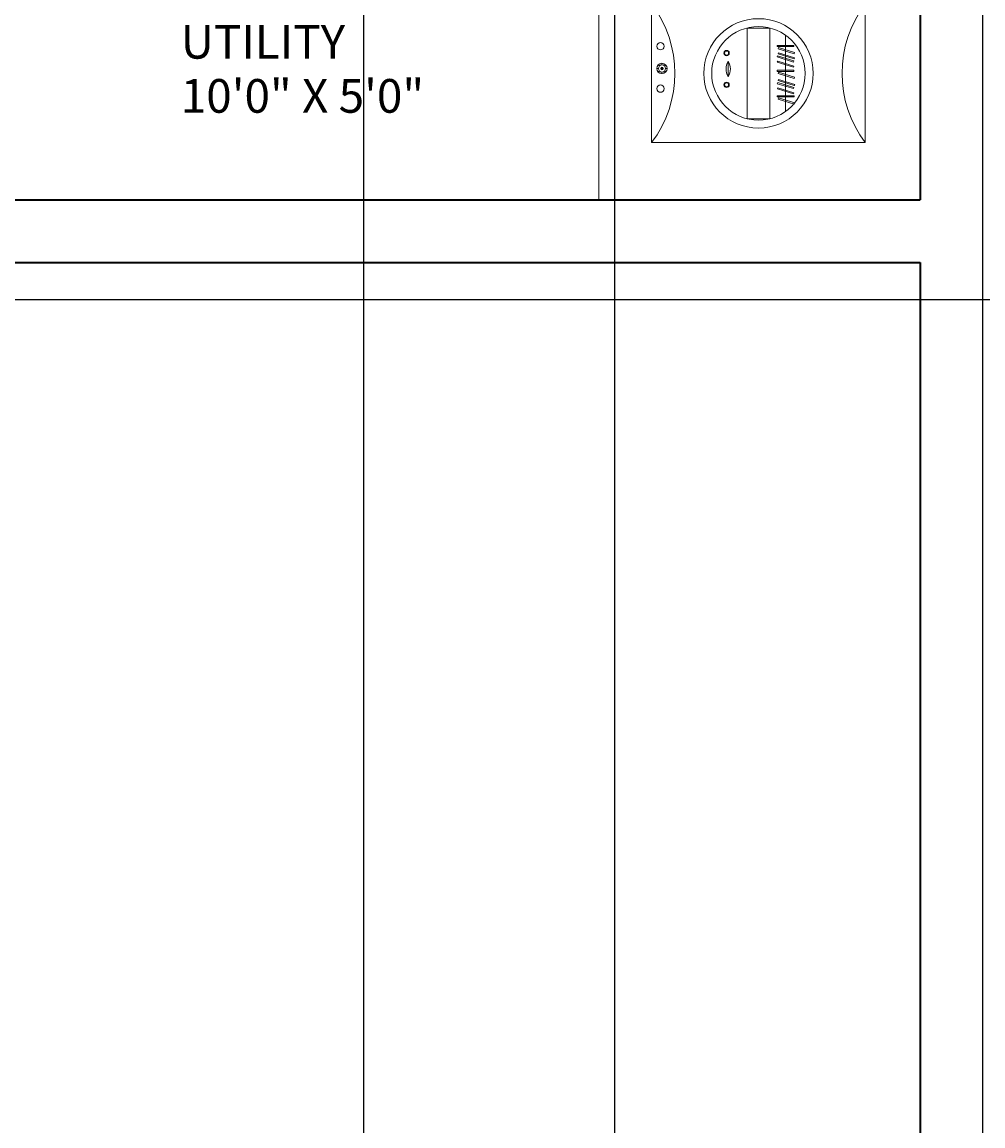
# Model space of a CAD drawing. Units: inches. Extents: x -61 to 1599, y -1316 to 257.
# Tile 81 of 204: x 407 to 545, y -565 to -407. Entities that reach past the tile are written whole.
import ezdxf

# ---------------------------------------------------------------- set-up
doc = ezdxf.new("R2010")
doc.units = ezdxf.units.IN
doc.header["$MEASUREMENT"] = 0
for name, color, linetype, lineweight in [('A-ANNO-DIMS', 2, 'Continuous', 18), ('A-AREA-IDEN', 1, 'Continuous', 18), ('A-EQPM', 9, 'Continuous', 18), ('A-FLOR-CASE', 8, 'Continuous', 18), ('WALLS', 4, 'Continuous', 35)]:
    doc.layers.add(name, color=color, linetype=linetype, lineweight=lineweight)
doc.styles.get("Standard").update_dxf_attribs({"font": 'arial.ttf'})
doc.dimstyles.get("Standard").update_dxf_attribs({"dimtxt": 0.18, "dimasz": 0.18, "dimexe": 0.18, "dimexo": 0.0625, "dimgap": 0.09, "dimtad": 0, "dimtih": 1, "dimtoh": 1, "dimdec": 0, "dimzin": 0, "dimdsep": 46, "dimlunit": 3, "dimtxsty": 'Standard', "dimcen": 0.09, "dimadec": 0, "dimazin": 0, "dimtfac": 1, "dimtdec": 0, "dimtofl": 0, "dimtmove": 0, "dimatfit": 3, "dimfxl": 1, "dimtolj": 1, "dimtzin": 0, "dimarcsym": 0})

# ---------------------------------------------------------------- blocks, each defined once
blk = doc.blocks.new('WASHING-MACHINE')
for p, q in [((19.24, 4.47), (19.22, 15.41)), ((0.96, 11.16), (1.13, 11)), ((1.49, 11.38), (1.49, 11.15)), ((2.02, 11.15), (1.86, 10.99)), ((11, 9.47), (11, 11.68)), ((0.98, 10.64), (0.75, 10.64)), ((1.12, 10.28), (0.96, 10.12)), ((1.49, 10.12), (1.49, 9.89)), ((1.86, 10.28), (2.02, 10.12)), ((2.23, 10.64), (2, 10.64))]:
    blk.add_line(p, q)
for points in [[(30.68, 0), (0, 0), (0, 19.87), (30.68, 19.87)], [(16.98, 3.42), (13.7, 3.42), (13.7, 16.45), (16.98, 16.45)], [(20.43, 13.78), (18.01, 13.78), (18.01, 13.95), (20.43, 13.95)], [(18.21, 13.64), (20.52, 12.92), (20.47, 12.76), (18.16, 13.47)], [(18.22, 12.89), (20.53, 12.18), (20.48, 12.01), (18.17, 12.73)], [(18.09, 12.45), (20.41, 11.74), (20.35, 11.57), (18.04, 12.29)], [(18.1, 11.71), (20.41, 10.99), (20.36, 10.83), (18.05, 11.54)], [(20.44, 10.23), (18.02, 10.23), (18.02, 10.4), (20.44, 10.4)], [(18.22, 10.09), (20.53, 9.38), (20.48, 9.21), (18.17, 9.92)], [(18.1, 8.63), (20.42, 7.91), (20.37, 7.75), (18.05, 8.46)], [(18.23, 9.07), (20.54, 8.36), (20.49, 8.19), (18.18, 8.91)], [(20.45, 6.56), (18.03, 6.56), (18.03, 6.73), (20.45, 6.73)], [(18.11, 7.88), (20.42, 7.17), (20.37, 7), (18.06, 7.72)], [(18.23, 6.42), (20.54, 5.7), (20.49, 5.54), (18.18, 6.25)]]:
    blk.add_lwpolyline(points, close=True)
for centre, radius in [((15.34, 9.94), 7.85), ((15.34, 9.94), 7.85), ((15.34, 9.94), 6.71), ((1.28, 13.83), 0.526), ((10.77, 12.86), 0.381), ((10.77, 12.86), 0.289), ((1.49, 10.64), 0.742), ((1.49, 10.64), 0.513), ((1.49, 10.64), 0.178), ((1.49, 10.64), 0.07), ((1.28, 7.75), 0.526), ((10.77, 8.29), 0.381), ((10.77, 8.29), 0.289)]:
    blk.add_circle(centre, radius)
for centre, radius, start, end in [((-13.12, 9.94), 16.46, 322.8671, 37.1329), ((43.8, 9.94), 16.46, 142.8671, 217.1329), ((12.8, 10.57), 2.11, 148.4251, 211.5749), ((9.2, 10.57), 2.11, 328.4251, 31.5749)]:
    blk.add_arc(centre, radius, start, end)
blk = doc.blocks.new('*D699')
at = {"layer": 'A-ANNO-DIMS', "color": 0, "lineweight": -2, "transparency": 16777216}
for p, q in [((835.64, -167.17), (-61.08, -167.17)), ((-60.9, -167.35), (-60.9, -306.73)), ((-60.9, -446.47), (-60.9, -307.09)), ((841.64, -446.65), (-61.08, -446.65))]:
    blk.add_line(p, q, dxfattribs=at)
at = {"layer": 'A-ANNO-DIMS', "color": 0, "transparency": 16777216}
for points in [[(-60.93, -167.35), (-60.87, -167.35), (-60.9, -167.17)], [(-60.93, -446.47), (-60.87, -446.47), (-60.9, -446.65)]]:
    blk.add_solid(points, dxfattribs=at)
at = {"layer": 'DEFPOINTS', "color": 0, "transparency": 16777216}
for p in [(835.7, -167.17), (-60.9, -446.65), (841.7, -446.65)]:
    blk.add_point(p, dxfattribs=at)
at = {"layer": 'A-ANNO-DIMS', "color": 0, "transparency": 16777216, "insert": (-60.9, -306.91), "char_height": 0.18, "attachment_point": 5}
blk.add_mtext('\\A1;279.5', dxfattribs=at)
blk = doc.blocks.new('*D703')
at = {"layer": 'A-ANNO-DIMS', "color": 0, "lineweight": -2, "transparency": 16777216}
for p, q in [((372.32, -616.88), (372.32, 257.46)), ((372.5, 257.28), (413.7, 257.28)), ((455.65, 257.28), (414.45, 257.28)), ((455.83, -616.88), (455.83, 257.46))]:
    blk.add_line(p, q, dxfattribs=at)
at = {"layer": 'A-ANNO-DIMS', "color": 0, "transparency": 16777216}
for points in [[(372.5, 257.31), (372.5, 257.25), (372.32, 257.28)], [(455.65, 257.31), (455.65, 257.25), (455.83, 257.28)]]:
    blk.add_solid(points, dxfattribs=at)
at = {"layer": 'DEFPOINTS', "color": 0, "transparency": 16777216}
for p in [(455.83, 257.28), (372.32, -616.94), (455.83, -616.94)]:
    blk.add_point(p, dxfattribs=at)
at = {"layer": 'A-ANNO-DIMS', "color": 0, "transparency": 16777216, "insert": (414.08, 257.28), "char_height": 0.18, "attachment_point": 5}
blk.add_mtext('\\A1;83.51', dxfattribs=at)
blk = doc.blocks.new('*D704')
at = {"layer": 'A-ANNO-DIMS', "color": 0, "lineweight": -2, "transparency": 16777216}
for p, q in [((491.83, -616.88), (491.83, 257.46)), ((492.01, 257.28), (517.87, 257.28)), ((544.52, 257.28), (518.66, 257.28)), ((544.7, -616.88), (544.7, 257.46))]:
    blk.add_line(p, q, dxfattribs=at)
at = {"layer": 'A-ANNO-DIMS', "color": 0, "transparency": 16777216}
for points in [[(492.01, 257.31), (492.01, 257.25), (491.83, 257.28)], [(544.52, 257.31), (544.52, 257.25), (544.7, 257.28)]]:
    blk.add_solid(points, dxfattribs=at)
at = {"layer": 'DEFPOINTS', "color": 0, "transparency": 16777216}
for p in [(544.7, 257.28), (491.83, -616.94), (544.7, -616.94)]:
    blk.add_point(p, dxfattribs=at)
at = {"layer": 'A-ANNO-DIMS', "color": 0, "transparency": 16777216, "insert": (518.27, 257.28), "char_height": 0.18, "attachment_point": 5}
blk.add_mtext('\\A1;52.87', dxfattribs=at)

msp = doc.modelspace()

# ---------------------------------------------------------------- linework, layer by layer
at = {"layer": 'A-FLOR-CASE'}
msp.add_line((489.5747, -432.3229), (489.5747, -378.3229), dxfattribs=at)
at = {"layer": 'WALLS'}
for p, q in [((535.7028, -378.3229), (535.7028, -432.3229)), ((403.7028, -432.3229), (535.7028, -432.3229)), ((403.7028, -441.3229), (535.7028, -441.3229)), ((535.7028, -441.3229), (535.7028, -567.169)), ((535.7028, -561.169), (535.7028, -741.169))]:
    msp.add_line(p, q, dxfattribs=at)

# ---------------------------------------------------------------- block references
at = {"layer": 'A-EQPM'}
msp.add_blockref('WASHING-MACHINE', (497.133, -424.099), dxfattribs=at)

# ---------------------------------------------------------------- texts
at = {"layer": 'A-AREA-IDEN'}
for s, height, p in [('UTILITY', 4.8321, (429.5332, -412.0454)), ('10\'0" X 5\'0"', 4.832098, (429.5332, -419.8078))]:
    msp.add_text(s, height=height, dxfattribs=at).set_placement(p)

# ---------------------------------------------------------------- dimensions: what is measured, and where the dimension line sits
at = {"layer": 'A-ANNO-DIMS'}
for base, p1, p2, picture, middle in [((455.8327, 257.2771), (372.3201, -616.9446), (455.8327, -616.9446), '*D703', (414.0764, 257.2771)), ((544.7028, 257.2771), (491.8327, -616.9446), (544.7028, -616.9446), '*D704', (518.2677, 257.2771))]:
    dim = msp.add_linear_dim(base=base, p1=p1, p2=p2, dimstyle='Standard', override={"dimdec": 2, "dimlfac": 1, "dimrnd": 0, "dimzin": 0, "dimdsep": 46, "dimlunit": 2}, dxfattribs=at)
    dim.commit()
    dim.dimension.update_dxf_attribs({"geometry": picture, "text_midpoint": middle})
dim = msp.add_linear_dim(base=(-60.8972, -446.6462), p1=(835.7028, -167.169), p2=(841.7028, -446.6462), angle=90, dimstyle='Standard', override={"dimdec": 1, "dimlfac": 1, "dimrnd": 0, "dimzin": 0, "dimdsep": 46, "dimlunit": 2}, dxfattribs=at)
dim.commit()
dim.dimension.update_dxf_attribs({"geometry": '*D699', "text_midpoint": (-60.8972, -306.9076)})

doc.saveas('drawing.dxf')
